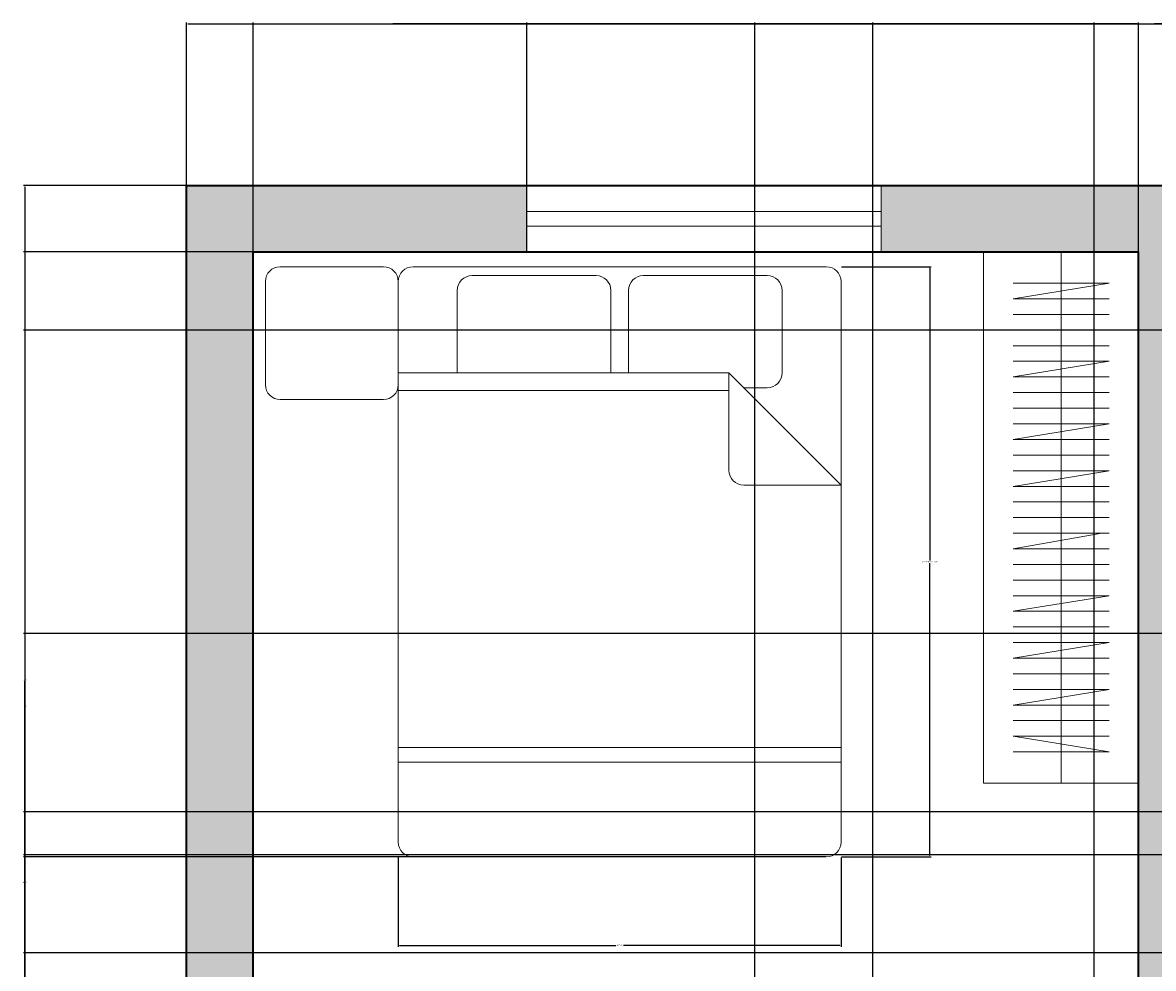
# Model space of a CAD drawing. Units: inches. Extents: x 2800 to 3283, y 1752 to 2114.
# Tile 3 of 6: x 2800 to 2954, y 1986 to 2114. Entities that reach past the tile are written whole.
import ezdxf

# ---------------------------------------------------------------- set-up
doc = ezdxf.new("R2010")
doc.units = ezdxf.units.IN
for name, color, linetype, lineweight in [('A-ANNO-DIMS', 2, 'Continuous', 18), ('A-FLOR-CASE', 8, 'Continuous', 18), ('A-FURN', 9, 'Continuous', 18), ('A-GLAZ', 4, 'Continuous', 18), ('A-WALL', 7, 'Continuous', 35)]:
    doc.layers.add(name, color=color, linetype=linetype, lineweight=lineweight)
doc.layers.add('A-WALL-PATT', color=18, linetype='Continuous', lineweight=13, true_color=0x000000)
doc.styles.get("Standard").update_dxf_attribs({"font": 'arial.ttf'})
doc.dimstyles.get("Standard").update_dxf_attribs({"dimtxt": 0.18, "dimasz": 0.18, "dimexe": 0.18, "dimexo": 0.0625, "dimgap": 0.09, "dimtad": 0, "dimtih": 1, "dimtoh": 1, "dimdec": 4, "dimzin": 0, "dimdsep": 46, "dimtxsty": 'Standard', "dimcen": 0.09, "dimadec": 0, "dimazin": 0, "dimtfac": 1, "dimtdec": 4, "dimtofl": 0, "dimtmove": 0, "dimatfit": 3, "dimfxl": 1, "dimtolj": 1, "dimtzin": 0, "dimarcsym": 0})

# ---------------------------------------------------------------- blocks, each defined once
blk = doc.blocks.new('Bed - Queen')
for p, q in [((2, 0), (58, 0)), ((10, -1.2), (26.8, -1.2)), ((33.2, -1.2), (50, -1.2)), ((0, -78), (0, -2)), ((60, -2), (60, -78)), ((8, -14.4), (8, -3.2)), ((28.8, -3.2), (28.8, -14.4)), ((31.2, -14.4), (31.2, -3.2)), ((52, -3.2), (52, -14.4)), ((0, -14.4), (44.8, -14.4)), ((60, -29.6), (44.8, -14.4)), ((44.8, -14.4), (44.8, -27.6)), ((44.8, -16.8), (0, -16.8)), ((50, -16.4), (46.8, -16.4)), ((46.8, -29.6), (60, -29.6)), ((0, -65.18), (60, -65.18)), ((0, -67.18), (60, -67.18)), ((58, -80), (2, -80))]:
    blk.add_line(p, q)
for centre, start, end in [((58, -2), 0, 90), ((2, -2), 90, 180), ((10, -3.2), 90, 180), ((26.8, -3.2), 0, 90), ((33.2, -3.2), 90, 180), ((50, -3.2), 0, 90), ((50, -14.4), 270, 0), ((46.8, -27.6), 180, 270), ((2, -78), 180, 270), ((58, -78), 270, 0)]:
    blk.add_arc(centre, 2, start, end)
blk = doc.blocks.new('WARDROBE-72')
for p, q in [((10.5, 72), (10.5, 0)), ((17, 63.53), (4, 63.53)), ((17, 61.41), (4, 61.41)), ((17, 59.29), (4, 59.29)), ((17, 52.94), (4, 52.94)), ((17, 50.82), (4, 50.82)), ((17, 44.47), (4, 44.47)), ((17, 38.12), (4, 38.12)), ((17, 36), (4, 36)), ((17, 33.88), (4, 33.88)), ((17, 29.65), (4, 29.65)), ((17, 27.53), (4, 27.53)), ((17, 21.18), (4, 21.18)), ((17, 14.82), (4, 14.82)), ((17, 8.47), (4, 8.47))]:
    blk.add_line(p, q)
for points in [[(0, 0), (0, 72), (21, 72), (21, 0), (0, 0), (21, 0)], [(4, 67.76), (17, 67.76), (4, 65.65), (17, 65.65)], [(4, 57.18), (17, 57.18), (4, 55.06), (17, 55.06)], [(4, 48.71), (17, 48.71), (4, 46.59), (17, 46.59)], [(4, 42.35), (17, 42.35), (4, 40.23), (17, 40.23)], [(16.02, 33.88), (4, 31.76), (17, 31.76)], [(4, 25.41), (17, 25.41), (4, 23.29), (17, 23.29)], [(4, 19.06), (17, 19.06), (4, 16.94), (17, 16.94)], [(4, 12.71), (17, 12.71), (4, 10.59), (17, 10.59)], [(4, 4.23), (17, 4.23), (4, 6.35), (17, 6.35)]]:
    blk.add_lwpolyline(points)
blk = doc.blocks.new('WIN-48')
for p, q in [((0, 5.5), (48, 5.5)), ((0, 3.5), (48, 3.5))]:
    blk.add_line(p, q)
for points in [[(0, 0), (0, 9)], [(48, 9), (48, 0)]]:
    blk.add_lwpolyline(points)
blk = doc.blocks.new('*D23')
at = {"layer": 'A-ANNO-DIMS', "color": 0, "lineweight": -2, "transparency": 16777216}
for p, q in [((2911.29, 2081.27), (2923.41, 2081.27)), ((2923.23, 2081.09), (2923.23, 2041.46)), ((2923.23, 2001.45), (2923.23, 2041.08)), ((2911.29, 2001.27), (2923.41, 2001.27))]:
    blk.add_line(p, q, dxfattribs=at)
at = {"layer": 'A-ANNO-DIMS', "color": 0, "transparency": 16777216}
for points in [[(2923.2, 2081.09), (2923.26, 2081.09), (2923.23, 2081.27)], [(2923.2, 2001.45), (2923.26, 2001.45), (2923.23, 2001.27)]]:
    blk.add_solid(points, dxfattribs=at)
at = {"layer": 'Defpoints', "color": 0, "transparency": 16777216}
for p in [(2911.23, 2081.27), (2923.23, 2081.27), (2911.23, 2001.27)]:
    blk.add_point(p, dxfattribs=at)
at = {"layer": 'A-ANNO-DIMS', "color": 0, "transparency": 16777216, "insert": (2923.23, 2041.27), "char_height": 0.18, "attachment_point": 5}
blk.add_mtext('\\A1;QUEEN BED 80 TYP.', dxfattribs=at)
blk = doc.blocks.new('*D24')
at = {"layer": 'A-ANNO-DIMS', "color": 0, "lineweight": -2, "transparency": 16777216}
for p, q in [((2851.23, 2001.21), (2851.23, 1989.09)), ((2911.23, 2001.21), (2911.23, 1989.09)), ((2851.41, 1989.27), (2880.7, 1989.27)), ((2911.05, 1989.27), (2881.75, 1989.27))]:
    blk.add_line(p, q, dxfattribs=at)
at = {"layer": 'A-ANNO-DIMS', "color": 0, "transparency": 16777216}
for points in [[(2851.41, 1989.3), (2851.41, 1989.24), (2851.23, 1989.27)], [(2911.05, 1989.3), (2911.05, 1989.24), (2911.23, 1989.27)]]:
    blk.add_solid(points, dxfattribs=at)
at = {"layer": 'Defpoints', "color": 0, "transparency": 16777216}
for p in [(2851.23, 2001.27), (2911.23, 2001.27), (2911.23, 1989.27)]:
    blk.add_point(p, dxfattribs=at)
at = {"layer": 'A-ANNO-DIMS', "color": 0, "transparency": 16777216, "insert": (2881.23, 1989.27), "char_height": 0.18, "attachment_point": 5}
blk.add_mtext('\\A1;60 TYP.', dxfattribs=at)
blk = doc.blocks.new('*D43')
at = {"layer": 'A-ANNO-DIMS', "color": 0, "lineweight": -2, "transparency": 16777216}
for p, q in [((2822.54, 2092.33), (2822.54, 2114.36)), ((2822.72, 2114.18), (3041.25, 2114.18)), ((3260.36, 2114.18), (3041.84, 2114.18)), ((3260.54, 2092.33), (3260.54, 2114.36))]:
    blk.add_line(p, q, dxfattribs=at)
at = {"layer": 'A-ANNO-DIMS', "color": 0, "transparency": 16777216}
for points in [[(2822.72, 2114.21), (2822.72, 2114.15), (2822.54, 2114.18)], [(3260.36, 2114.21), (3260.36, 2114.15), (3260.54, 2114.18)]]:
    blk.add_solid(points, dxfattribs=at)
at = {"layer": 'Defpoints', "color": 0, "transparency": 16777216}
for p in [(3260.54, 2114.18), (2822.54, 2092.27), (3260.54, 2092.27)]:
    blk.add_point(p, dxfattribs=at)
at = {"layer": 'A-ANNO-DIMS', "color": 0, "transparency": 16777216, "insert": (3041.54, 2114.18), "char_height": 0.18, "attachment_point": 5}
blk.add_mtext('\\A1;438', dxfattribs=at)
blk = doc.blocks.new('*D44')
at = {"layer": 'A-ANNO-DIMS', "color": 0, "lineweight": -2, "transparency": 16777216}
for p, q in [((2822.48, 2092.27), (2800.45, 2092.27)), ((2800.63, 2092.09), (2800.63, 1933.45)), ((2800.63, 1774.45), (2800.63, 1933.09)), ((2822.48, 1774.27), (2800.45, 1774.27))]:
    blk.add_line(p, q, dxfattribs=at)
at = {"layer": 'A-ANNO-DIMS', "color": 0, "transparency": 16777216}
for points in [[(2800.6, 2092.09), (2800.66, 2092.09), (2800.63, 2092.27)], [(2800.6, 1774.45), (2800.66, 1774.45), (2800.63, 1774.27)]]:
    blk.add_solid(points, dxfattribs=at)
at = {"layer": 'Defpoints', "color": 0, "transparency": 16777216}
for p in [(2800.63, 2092.27), (2822.54, 2092.27), (2822.54, 1774.27)]:
    blk.add_point(p, dxfattribs=at)
at = {"layer": 'A-ANNO-DIMS', "color": 0, "transparency": 16777216, "insert": (2800.63, 1933.27), "char_height": 0.18, "attachment_point": 5}
blk.add_mtext('\\A1;318', dxfattribs=at)
blk = doc.blocks.new('*D45')
at = {"layer": 'A-ANNO-DIMS', "color": 0, "lineweight": -2, "transparency": 16777216}
for p, q in [((2831.54, 1967.33), (2831.54, 2114.36)), ((2831.72, 2114.18), (2891.26, 2114.18)), ((2951.36, 2114.18), (2891.82, 2114.18)), ((2951.54, 1967.33), (2951.54, 2114.36))]:
    blk.add_line(p, q, dxfattribs=at)
at = {"layer": 'A-ANNO-DIMS', "color": 0, "transparency": 16777216}
for points in [[(2831.72, 2114.21), (2831.72, 2114.15), (2831.54, 2114.18)], [(2951.36, 2114.21), (2951.36, 2114.15), (2951.54, 2114.18)]]:
    blk.add_solid(points, dxfattribs=at)
at = {"layer": 'Defpoints', "color": 0, "transparency": 16777216}
for p in [(2951.54, 2114.18), (2831.54, 1967.27), (2951.54, 1967.27)]:
    blk.add_point(p, dxfattribs=at)
at = {"layer": 'A-ANNO-DIMS', "color": 0, "transparency": 16777216, "insert": (2891.54, 2114.18), "char_height": 0.18, "attachment_point": 5}
blk.add_mtext('\\A1;120', dxfattribs=at)
blk = doc.blocks.new('*D46')
at = {"layer": 'A-ANNO-DIMS', "color": 0, "lineweight": -2, "transparency": 16777216}
for p, q in [((2951.54, 2083.33), (2951.54, 2114.36)), ((2951.72, 2114.18), (2953.39, 2114.18)), ((2955.36, 2114.18), (2953.7, 2114.18)), ((2955.54, 2083.33), (2955.54, 2114.36))]:
    blk.add_line(p, q, dxfattribs=at)
at = {"layer": 'A-ANNO-DIMS', "color": 0, "transparency": 16777216}
for points in [[(2951.72, 2114.21), (2951.72, 2114.15), (2951.54, 2114.18)], [(2955.36, 2114.21), (2955.36, 2114.15), (2955.54, 2114.18)]]:
    blk.add_solid(points, dxfattribs=at)
at = {"layer": 'Defpoints', "color": 0, "transparency": 16777216}
for p in [(2955.54, 2114.18), (2951.54, 2083.27), (2955.54, 2083.27)]:
    blk.add_point(p, dxfattribs=at)
at = {"layer": 'A-ANNO-DIMS', "color": 0, "transparency": 16777216, "insert": (2953.54, 2114.18), "char_height": 0.18, "attachment_point": 5}
blk.add_mtext('\\A1;4', dxfattribs=at)
blk = doc.blocks.new('*D49')
at = {"layer": 'A-ANNO-DIMS', "color": 0, "lineweight": -2, "transparency": 16777216}
for p, q in [((2831.48, 2083.27), (2800.45, 2083.27)), ((2800.63, 2083.09), (2800.63, 2025.45)), ((2800.63, 1967.45), (2800.63, 2025.09)), ((2831.48, 1967.27), (2800.45, 1967.27))]:
    blk.add_line(p, q, dxfattribs=at)
at = {"layer": 'A-ANNO-DIMS', "color": 0, "transparency": 16777216}
for points in [[(2800.6, 2083.09), (2800.66, 2083.09), (2800.63, 2083.27)], [(2800.6, 1967.45), (2800.66, 1967.45), (2800.63, 1967.27)]]:
    blk.add_solid(points, dxfattribs=at)
at = {"layer": 'Defpoints', "color": 0, "transparency": 16777216}
for p in [(2800.63, 2083.27), (2831.54, 2083.27), (2831.54, 1967.27)]:
    blk.add_point(p, dxfattribs=at)
at = {"layer": 'A-ANNO-DIMS', "color": 0, "transparency": 16777216, "insert": (2800.63, 2025.27), "char_height": 0.18, "attachment_point": 5}
blk.add_mtext('\\A1;116', dxfattribs=at)
blk = doc.blocks.new('*D54')
at = {"layer": 'A-ANNO-DIMS', "color": 0, "lineweight": -2, "transparency": 16777216}
for p, q in [((2831.54, 1903.33), (2831.54, 2114.36)), ((2831.72, 2114.18), (2865.32, 2114.18)), ((2899.36, 2114.18), (2865.76, 2114.18)), ((2899.54, 1903.33), (2899.54, 2114.36))]:
    blk.add_line(p, q, dxfattribs=at)
at = {"layer": 'A-ANNO-DIMS', "color": 0, "transparency": 16777216}
for points in [[(2831.72, 2114.21), (2831.72, 2114.15), (2831.54, 2114.18)], [(2899.36, 2114.21), (2899.36, 2114.15), (2899.54, 2114.18)]]:
    blk.add_solid(points, dxfattribs=at)
at = {"layer": 'Defpoints', "color": 0, "transparency": 16777216}
for p in [(2899.54, 2114.18), (2831.54, 1903.27), (2899.54, 1903.27)]:
    blk.add_point(p, dxfattribs=at)
at = {"layer": 'A-ANNO-DIMS', "color": 0, "transparency": 16777216, "insert": (2865.54, 2114.18), "char_height": 0.18, "attachment_point": 5}
blk.add_mtext('\\A1;68', dxfattribs=at)
blk = doc.blocks.new('*D56')
at = {"layer": 'A-ANNO-DIMS', "color": 0, "lineweight": -2, "transparency": 16777216}
for p, q in [((2831.54, 2083.33), (2831.54, 2114.36)), ((2831.72, 2114.18), (2849.71, 2114.18)), ((2868.48, 2114.18), (2850.5, 2114.18)), ((2868.66, 2083.33), (2868.66, 2114.36))]:
    blk.add_line(p, q, dxfattribs=at)
at = {"layer": 'A-ANNO-DIMS', "color": 0, "transparency": 16777216}
for points in [[(2831.72, 2114.21), (2831.72, 2114.15), (2831.54, 2114.18)], [(2868.48, 2114.21), (2868.48, 2114.15), (2868.66, 2114.18)]]:
    blk.add_solid(points, dxfattribs=at)
at = {"layer": 'Defpoints', "color": 0, "transparency": 16777216}
for p in [(2868.66, 2114.18), (2831.54, 2083.27), (2868.66, 2083.27)]:
    blk.add_point(p, dxfattribs=at)
at = {"layer": 'A-ANNO-DIMS', "color": 0, "transparency": 16777216, "insert": (2850.1, 2114.18), "char_height": 0.18, "attachment_point": 5}
blk.add_mtext('\\A1;37.12', dxfattribs=at)
blk = doc.blocks.new('*D66')
at = {"layer": 'A-ANNO-DIMS', "color": 0, "lineweight": -2, "transparency": 16777216}
for p, q in [((2915.54, 1899.33), (2915.54, 2114.36)), ((2915.72, 2114.18), (2930.32, 2114.18)), ((2945.36, 2114.18), (2930.76, 2114.18)), ((2945.54, 1899.33), (2945.54, 2114.36))]:
    blk.add_line(p, q, dxfattribs=at)
at = {"layer": 'A-ANNO-DIMS', "color": 0, "transparency": 16777216}
for points in [[(2915.72, 2114.21), (2915.72, 2114.15), (2915.54, 2114.18)], [(2945.36, 2114.21), (2945.36, 2114.15), (2945.54, 2114.18)]]:
    blk.add_solid(points, dxfattribs=at)
at = {"layer": 'Defpoints', "color": 0, "transparency": 16777216}
for p in [(2945.54, 2114.18), (2915.54, 1899.27), (2945.54, 1899.27)]:
    blk.add_point(p, dxfattribs=at)
at = {"layer": 'A-ANNO-DIMS', "color": 0, "transparency": 16777216, "insert": (2930.54, 2114.18), "char_height": 0.18, "attachment_point": 5}
blk.add_mtext('\\A1;30', dxfattribs=at)
blk = doc.blocks.new('*D67')
at = {"layer": 'A-ANNO-DIMS', "color": 0, "lineweight": -2, "transparency": 16777216}
for p, q in [((2945.54, 1899.33), (2945.54, 2114.36)), ((2945.72, 2114.18), (2948.39, 2114.18)), ((2951.36, 2114.18), (2948.69, 2114.18)), ((2951.54, 1899.33), (2951.54, 2114.36))]:
    blk.add_line(p, q, dxfattribs=at)
at = {"layer": 'A-ANNO-DIMS', "color": 0, "transparency": 16777216}
for points in [[(2945.72, 2114.21), (2945.72, 2114.15), (2945.54, 2114.18)], [(2951.36, 2114.21), (2951.36, 2114.15), (2951.54, 2114.18)]]:
    blk.add_solid(points, dxfattribs=at)
at = {"layer": 'Defpoints', "color": 0, "transparency": 16777216}
for p in [(2951.54, 2114.18), (2945.54, 1899.27), (2951.54, 1899.27)]:
    blk.add_point(p, dxfattribs=at)
at = {"layer": 'A-ANNO-DIMS', "color": 0, "transparency": 16777216, "insert": (2948.54, 2114.18), "char_height": 0.18, "attachment_point": 5}
blk.add_mtext('\\A1;6', dxfattribs=at)
blk = doc.blocks.new('*D77')
at = {"layer": 'A-ANNO-DIMS', "color": 0, "lineweight": -2, "transparency": 16777216}
for p, q in [((3076.62, 2072.66), (2800.45, 2072.66)), ((2800.63, 2072.48), (2800.63, 2021.84)), ((2800.63, 1970.84), (2800.63, 2021.48)), ((3076.62, 1970.66), (2800.45, 1970.66))]:
    blk.add_line(p, q, dxfattribs=at)
at = {"layer": 'A-ANNO-DIMS', "color": 0, "transparency": 16777216}
for points in [[(2800.6, 2072.48), (2800.66, 2072.48), (2800.63, 2072.66)], [(2800.6, 1970.84), (2800.66, 1970.84), (2800.63, 1970.66)]]:
    blk.add_solid(points, dxfattribs=at)
at = {"layer": 'Defpoints', "color": 0, "transparency": 16777216}
for p in [(3076.68, 2072.66), (2800.63, 1970.66), (3076.68, 1970.66)]:
    blk.add_point(p, dxfattribs=at)
at = {"layer": 'A-ANNO-DIMS', "color": 0, "transparency": 16777216, "insert": (2800.63, 2021.66), "char_height": 0.18, "attachment_point": 5}
blk.add_mtext('\\A1;102', dxfattribs=at)
blk = doc.blocks.new('*D80')
at = {"layer": 'A-ANNO-DIMS', "color": 0, "lineweight": -2, "transparency": 16777216}
for p, q in [((3045.08, 2031.54), (2800.45, 2031.54)), ((2800.63, 2031.36), (2800.63, 2016.73)), ((2800.63, 2001.72), (2800.63, 2016.36)), ((3045.08, 2001.54), (2800.45, 2001.54))]:
    blk.add_line(p, q, dxfattribs=at)
at = {"layer": 'A-ANNO-DIMS', "color": 0, "transparency": 16777216}
for points in [[(2800.6, 2031.36), (2800.66, 2031.36), (2800.63, 2031.54)], [(2800.6, 2001.72), (2800.66, 2001.72), (2800.63, 2001.54)]]:
    blk.add_solid(points, dxfattribs=at)
at = {"layer": 'Defpoints', "color": 0, "transparency": 16777216}
for p in [(2800.63, 2031.54), (3045.14, 2031.54), (3045.14, 2001.54)]:
    blk.add_point(p, dxfattribs=at)
at = {"layer": 'A-ANNO-DIMS', "color": 0, "transparency": 16777216, "insert": (2800.63, 2016.54), "char_height": 0.18, "attachment_point": 5}
blk.add_mtext('\\A1;30', dxfattribs=at)
blk = doc.blocks.new('*D81')
at = {"layer": 'A-ANNO-DIMS', "color": 0, "lineweight": -2, "transparency": 16777216}
for p, q in [((2909.16, 2001.27), (2800.45, 2001.27)), ((2800.63, 2001.09), (2800.63, 1984.45)), ((2800.63, 1967.45), (2800.63, 1984.09)), ((2915.48, 1967.27), (2800.45, 1967.27))]:
    blk.add_line(p, q, dxfattribs=at)
at = {"layer": 'A-ANNO-DIMS', "color": 0, "transparency": 16777216}
for points in [[(2800.6, 2001.09), (2800.66, 2001.09), (2800.63, 2001.27)], [(2800.6, 1967.45), (2800.66, 1967.45), (2800.63, 1967.27)]]:
    blk.add_solid(points, dxfattribs=at)
at = {"layer": 'Defpoints', "color": 0, "transparency": 16777216}
for p in [(2800.63, 2001.27), (2909.23, 2001.27), (2915.54, 1967.27)]:
    blk.add_point(p, dxfattribs=at)
at = {"layer": 'A-ANNO-DIMS', "color": 0, "transparency": 16777216, "insert": (2800.63, 1984.27), "char_height": 0.18, "attachment_point": 5}
blk.add_mtext('\\A1;34', dxfattribs=at)
blk = doc.blocks.new('*D82')
at = {"layer": 'A-ANNO-DIMS', "color": 0, "lineweight": -2, "transparency": 16777216}
for p, q in [((3171.82, 2007.36), (2800.45, 2007.36)), ((2800.63, 2007.18), (2800.63, 1998)), ((2800.63, 1988.45), (2800.63, 1997.63)), ((3179.48, 1988.27), (2800.45, 1988.27))]:
    blk.add_line(p, q, dxfattribs=at)
at = {"layer": 'A-ANNO-DIMS', "color": 0, "transparency": 16777216}
for points in [[(2800.6, 2007.18), (2800.66, 2007.18), (2800.63, 2007.36)], [(2800.6, 1988.45), (2800.66, 1988.45), (2800.63, 1988.27)]]:
    blk.add_solid(points, dxfattribs=at)
at = {"layer": 'Defpoints', "color": 0, "transparency": 16777216}
for p in [(2800.63, 2007.36), (3171.89, 2007.36), (3179.54, 1988.27)]:
    blk.add_point(p, dxfattribs=at)
at = {"layer": 'A-ANNO-DIMS', "color": 0, "transparency": 16777216, "insert": (2800.63, 1997.81), "char_height": 0.18, "attachment_point": 5}
blk.add_mtext('\\A1;19.09', dxfattribs=at)

msp = doc.modelspace()

# ---------------------------------------------------------------- hatches: boundary and pattern name
at = {"layer": 'A-WALL-PATT'}
h = msp.add_hatch(color=256, dxfattribs=at)
h.dxf.hatch_style = 1
h.paths.add_polyline_path([(2868.6629, 2092.2695), (2822.5432, 2092.2695), (2822.5432, 1946.3547), (2831.5432, 1946.3547), (2831.5432, 1963.2695), (2899.5432, 1963.2695), (2899.5432, 1957.2695), (2903.5432, 1957.2695), (2903.5432, 1963.2695), (2915.5432, 1963.2695), (2915.5432, 1967.2695), (2831.5432, 1967.2695), (2831.5432, 2083.2695), (2868.6629, 2083.2695)])
h = msp.add_hatch(color=256, dxfattribs=at)
h.dxf.hatch_style = 1
h.paths.add_polyline_path([(3023.883, 2092.2695), (2916.6629, 2092.2695), (2916.6629, 2083.2695), (2951.5432, 2083.2695), (2951.5432, 2011.2695), (2951.5432, 1967.2695), (2945.5432, 1967.2695), (2945.5432, 1963.2695), (2955.5432, 1963.2695), (2955.5432, 2083.2695), (3023.883, 2083.2695)])

# ---------------------------------------------------------------- linework, layer by layer
at = {"layer": 'A-FURN'}
msp.add_lwpolyline([(2835.2258, 2081.2722), (2849.2258, 2081.2722, -0.41421356), (2851.2258, 2079.2722), (2851.2258, 2065.2722, -0.41421356), (2849.2258, 2063.2722), (2835.2258, 2063.2722, -0.41421356), (2833.2258, 2065.2722), (2833.2258, 2079.2722, -0.41421356)], format="xyb", close=True, dxfattribs=at)
at = {"layer": 'A-WALL'}
for p, q in [((2831.5432, 2083.2695), (2951.5432, 2083.2695)), ((2831.5432, 1967.2695), (2831.5432, 2083.2695)), ((2951.5432, 1967.2695), (2951.5432, 2083.2695))]:
    msp.add_line(p, q, dxfattribs=at)
msp.add_lwpolyline([(2967.5432, 1774.2695), (2822.5432, 1774.2695), (2822.5432, 2092.2695), (3260.5432, 2092.2695), (3260.5432, 1774.2695), (3015.5432, 1774.2695)], dxfattribs=at)

# ---------------------------------------------------------------- block references
at = {"layer": 'A-FLOR-CASE'}
msp.add_blockref('WARDROBE-72', (2930.543, 2011.27), dxfattribs=at)
at = {"layer": 'A-FURN'}
msp.add_blockref('Bed - Queen', (2851.2258, 2081.2722), dxfattribs=at)
at = {"layer": 'A-GLAZ'}
msp.add_blockref('WIN-48', (2868.663, 2083.27), dxfattribs=at)

# ---------------------------------------------------------------- dimensions: what is measured, and where the dimension line sits
at = {"layer": 'A-ANNO-DIMS'}
for base, p1, p2, override, picture, middle in [((3260.5432, 2114.1845), (2822.5432, 2092.2695), (3260.5432, 2092.2695), {"dimdec": 0, "dimlfac": 1, "dimrnd": 0, "dimzin": 0, "dimdsep": 46, "dimlunit": 2}, '*D43', (3041.5432, 2114.1845)), ((2951.5432, 2114.1845), (2831.5432, 1967.2695), (2951.5432, 1967.2695), {"dimdec": 0, "dimlfac": 1, "dimrnd": 0, "dimzin": 0, "dimdsep": 46, "dimlunit": 2}, '*D45', (2891.5432, 2114.1845)), ((2899.5432, 2114.1845), (2831.5432, 1903.2695), (2899.5432, 1903.2695), {"dimdec": 0, "dimlfac": 1, "dimrnd": 0, "dimzin": 0, "dimdsep": 46, "dimlunit": 2}, '*D54', (2865.5432, 2114.1845)), ((2868.6629, 2114.1845), (2831.5432, 2083.2695), (2868.6629, 2083.2695), {"dimdec": 2, "dimlfac": 1, "dimrnd": 0, "dimzin": 0, "dimdsep": 46, "dimlunit": 2}, '*D56', (2850.103, 2114.1845)), ((2945.5432, 2114.1845), (2915.5432, 1899.2695), (2945.5432, 1899.2695), {"dimdec": 0, "dimlfac": 1, "dimrnd": 0, "dimzin": 0, "dimdsep": 46, "dimlunit": 2}, '*D66', (2930.5432, 2114.1845)), ((2951.5432, 2114.1845), (2945.5432, 1899.2695), (2951.5432, 1899.2695), {"dimdec": 0, "dimlfac": 1, "dimrnd": 0, "dimzin": 0, "dimdsep": 46, "dimlunit": 2}, '*D67', (2948.5432, 2114.1845)), ((2955.5432, 2114.1845), (2951.5432, 2083.2695), (2955.5432, 2083.2695), {"dimdec": 0, "dimlfac": 1, "dimrnd": 0, "dimzin": 0, "dimdsep": 46, "dimlunit": 2}, '*D46', (2953.5432, 2114.1845))]:
    dim = msp.add_linear_dim(base=base, p1=p1, p2=p2, dimstyle='Standard', override=override, dxfattribs=at)
    dim.commit()
    dim.dimension.update_dxf_attribs({"geometry": picture, "text_midpoint": middle})
for base, p1, p2, override, picture, middle in [((2800.6282, 2092.2695), (2822.5432, 1774.2695), (2822.5432, 2092.2695), {"dimdec": 0, "dimlfac": 1, "dimrnd": 0, "dimzin": 0, "dimdsep": 46, "dimlunit": 2}, '*D44', (2800.6282, 1933.2695)), ((2800.6282, 2083.2695), (2831.5432, 1967.2695), (2831.5432, 2083.2695), {"dimdec": 0, "dimlfac": 1, "dimrnd": 0, "dimzin": 0, "dimdsep": 46, "dimlunit": 2}, '*D49', (2800.6282, 2025.2695)), ((2800.6282, 1970.661), (3076.6778, 2072.661), (3076.6778, 1970.661), {"dimdec": 0, "dimlfac": 1, "dimrnd": 0, "dimzin": 0, "dimdsep": 46, "dimlunit": 2}, '*D77', (2800.6282, 2021.661)), ((2800.6282, 2031.544), (3045.1406, 2001.544), (3045.1406, 2031.544), {"dimdec": 0, "dimlfac": 1, "dimrnd": 0, "dimzin": 0, "dimdsep": 46, "dimlunit": 2}, '*D80', (2800.6282, 2016.544)), ((2800.6282, 2007.3598), (3179.5432, 1988.2695), (3171.8868, 2007.3598), {"dimdec": 2, "dimlfac": 1, "dimrnd": 0, "dimzin": 0, "dimdsep": 46, "dimlunit": 2}, '*D82', (2800.6282, 1997.8147)), ((2800.6282, 2001.2722), (2915.5432, 1967.2695), (2909.2258, 2001.2722), {"dimdec": 0, "dimlfac": 1, "dimrnd": 0, "dimzin": 0, "dimdsep": 46, "dimlunit": 2}, '*D81', (2800.6282, 1984.2708))]:
    dim = msp.add_linear_dim(base=base, p1=p1, p2=p2, angle=90, dimstyle='Standard', override=override, dxfattribs=at)
    dim.commit()
    dim.dimension.update_dxf_attribs({"geometry": picture, "text_midpoint": middle})
dim = msp.add_linear_dim(base=(2923.2258, 2081.2722), p1=(2911.2258, 2001.2722), p2=(2911.2258, 2081.2722), angle=90, text='QUEEN BED <> TYP.', dimstyle='Standard', override={"dimdec": 0, "dimlfac": 1, "dimrnd": 0, "dimzin": 0, "dimdsep": 46, "dimlunit": 2}, dxfattribs=at)
dim.commit()
dim.dimension.update_dxf_attribs({"geometry": '*D23', "text_midpoint": (2923.2258, 2041.2722)})
dim = msp.add_linear_dim(base=(2911.2258, 1989.2722), p1=(2851.2258, 2001.2722), p2=(2911.2258, 2001.2722), text='<> TYP.', dimstyle='Standard', override={"dimdec": 0, "dimlfac": 1, "dimrnd": 0, "dimzin": 0, "dimdsep": 46, "dimlunit": 2}, dxfattribs=at)
dim.commit()
dim.dimension.update_dxf_attribs({"geometry": '*D24', "text_midpoint": (2881.2258, 1989.2722)})

doc.saveas('drawing.dxf')
